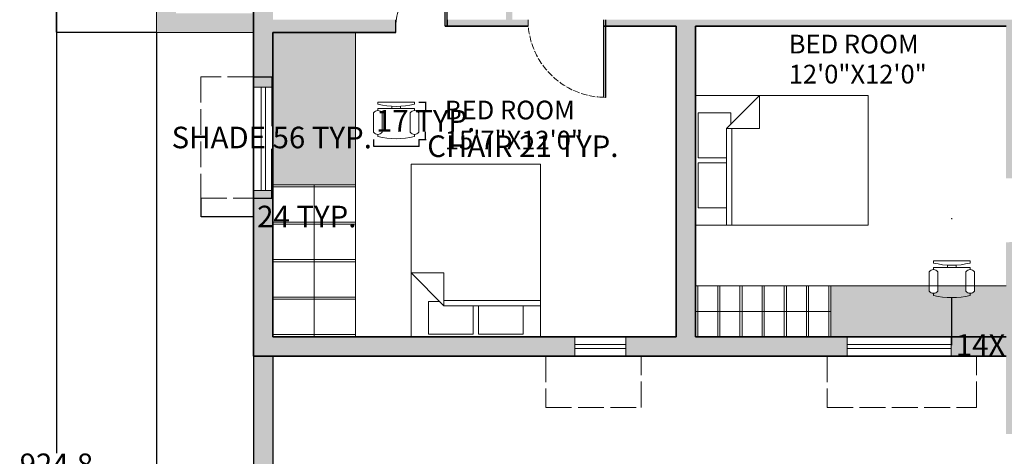
# Model space of a CAD drawing. Units: inches. Extents: x 215 to 969, y -612 to 418.
# Tile 4 of 8: x 227 to 684, y -93 to 109. Entities that reach past the tile are written whole.
import ezdxf

# ---------------------------------------------------------------- set-up
doc = ezdxf.new("R2010")
doc.units = ezdxf.units.IN
doc.header["$MEASUREMENT"] = 0
doc.linetypes.add('ACAD_ISO02W100', pattern=[15, 12, -3])
for name, color, linetype, lineweight in [('A-ANNO-DIMS', 2, 'Continuous', 18), ('A-AREA-IDEN', 7, 'Continuous', 18), ('A-DOOR', 3, 'Continuous', 25), ('A-DOOR-SWNG', 3, 'ACAD_ISO02W100', 13), ('A-FLOR-CASE', 9, 'Continuous', 18), ('A-FLOR-OVHD', 8, 'ACAD_ISO02W100', 13), ('A-FLOR-SHFT', 9, 'Continuous', 18), ('A-FLOR-SLAB', 7, 'Continuous', 25), ('A-FURN', 8, 'Continuous', 18), ('A-GLAZ', 4, 'Continuous', 18), ('A-WALL', 7, 'Continuous', 35)]:
    doc.layers.add(name, color=color, linetype=linetype, lineweight=lineweight)
doc.layers.add('A-WALL-PATT', color=252, linetype='Continuous', lineweight=13, true_color=0x939598)
doc.styles.get("Standard").update_dxf_attribs({"font": 'arial.ttf'})
doc.dimstyles.get("Standard").update_dxf_attribs({"dimtxt": 10, "dimasz": 0.18, "dimexe": 0.18, "dimexo": 0.0625, "dimgap": 0.09, "dimtad": 0, "dimtih": 1, "dimtoh": 1, "dimdec": 0, "dimzin": 0, "dimdsep": 46, "dimlunit": 3, "dimtxsty": 'Standard', "dimcen": 0.09, "dimadec": 0, "dimazin": 0, "dimtfac": 1, "dimtdec": 0, "dimtofl": 0, "dimtmove": 0, "dimatfit": 3, "dimfxl": 1, "dimtolj": 1, "dimtzin": 0, "dimarcsym": 0})

# ---------------------------------------------------------------- blocks, each defined once
blk = doc.blocks.new('Bed - Queen')
for p, q in [((0, -80.00003), (0, 0)), ((0, 0), (59.99999, 0)), ((59.99999, 0), (59.99999, -80.00003)), ((7.99999, -1.2), (28.79998, -1.2)), ((7.99999, -14.4), (7.99999, -1.2)), ((28.79998, -1.2), (28.79998, -14.4)), ((31.19999, -1.2), (51.99999, -1.2)), ((31.19999, -14.4), (31.19999, -1.2)), ((51.99999, -1.2), (51.99999, -16.4)), ((0, -14.4), (44.8, -14.4)), ((44.8, -16.8), (0, -16.8)), ((59.99999, -29.6), (44.8, -14.4)), ((44.8, -14.4), (44.8, -29.6)), ((51.99999, -16.4), (46.79936, -16.4)), ((44.8, -29.6), (59.99999, -29.6)), ((59.99999, -80.00003), (0, -80.00003))]:
    blk.add_line(p, q)
blk = doc.blocks.new('Chair - Desk')
for p, q in [((-8.5, 0), (-8.5, -1)), ((-8.5, 0), (8.5, 0)), ((8.5, 0), (8.5, -1)), ((-8.5, -3), (-8.5, -4)), ((-8.5, -3), (8.5, -3)), ((-2, -3), (-2, -1.9355)), ((2, -1.9576), (2, -3)), ((8.5, -3), (8.5, -4)), ((-10.5, -5), (-10.5, -14)), ((-6.5, -14), (-6.5, -5)), ((6.5, -5), (6.5, -14)), ((10.5, -14), (10.5, -5)), ((-8.5, -15), (-8.5, -16)), ((8.5, -15), (8.5, -16))]:
    blk.add_line(p, q)
for centre, radius, start, end in [((-8.5, -6.5), 2.5, 36.8699, 143.1301), ((0, 34.625), 36.625, 256.5803, 283.4197), ((8.5, -6.5), 2.5, 36.8699, 143.1301), ((-8.5, -12.5), 2.5, 216.8699, 323.1301), ((0, 19.625), 36.625, 256.5803, 283.4197), ((8.5, -12.5), 2.5, 216.8699, 323.1301)]:
    blk.add_arc(centre, radius, start, end)
blk = doc.blocks.new('WINDOW-SHADE-56')
for p, q in [((24.46, 56.34), (0, 56.34)), ((0, 56.34), (0, 0)), ((0, 0), (24.46, 0))]:
    blk.add_line(p, q)
blk = doc.blocks.new('WIN-FRAME-24A')
for p, q in [((0, 0), (0, 9)), ((23.77, 5.5), (0, 5.5)), ((23.77, 0), (23.77, 9)), ((0, 4.5), (0, 0)), ((23.77, 3.5), (0, 3.5))]:
    blk.add_line(p, q)
blk = doc.blocks.new('WIN-FRAME-48')
for p, q in [((0, 4.5), (0, 9)), ((0, 9), (0, 0)), ((48.04, 5.5), (0, 5.5)), ((48.04, 0), (48.04, 9)), ((48.04, 3.5), (0, 3.5))]:
    blk.add_line(p, q)
blk = doc.blocks.new('*D21')
at = {"layer": 'A-ANNO-DIMS', "color": 0, "lineweight": -2, "transparency": 16777216}
for p, q in [((391.01, 53.65), (391.01, 50.38)), ((391.19, 50.56), (411.83, 50.56)), ((412.01, 53.65), (412.01, 50.38)), ((412.01, 50.56), (412.19, 50.56))]:
    blk.add_line(p, q, dxfattribs=at)
at = {"layer": 'A-ANNO-DIMS', "color": 0, "transparency": 16777216}
for points in [[(391.19, 50.59), (391.19, 50.53), (391.01, 50.56)], [(411.83, 50.59), (411.83, 50.53), (412.01, 50.56)]]:
    blk.add_solid(points, dxfattribs=at)
at = {"layer": 'Defpoints', "color": 0, "transparency": 16777216}
for p in [(391.01, 53.71), (412.01, 53.71), (412.01, 50.56)]:
    blk.add_point(p, dxfattribs=at)
at = {"layer": 'A-ANNO-DIMS', "color": 0, "transparency": 16777216, "insert": (460.24, 50.56), "char_height": 10, "attachment_point": 5}
blk.add_mtext('\\A1;CHAIR 21 TYP.', dxfattribs=at)
blk = doc.blocks.new('*D22')
at = {"layer": 'A-ANNO-DIMS', "color": 0, "lineweight": -2, "transparency": 16777216}
for p, q in [((412.08, 71.05), (415.34, 71.05)), ((415.16, 70.87), (415.16, 67.49)), ((415.16, 53.89), (415.16, 57.27)), ((412.08, 53.71), (415.34, 53.71))]:
    blk.add_line(p, q, dxfattribs=at)
at = {"layer": 'A-ANNO-DIMS', "color": 0, "transparency": 16777216}
for points in [[(415.13, 70.87), (415.19, 70.87), (415.16, 71.05)], [(415.13, 53.89), (415.19, 53.89), (415.16, 53.71)]]:
    blk.add_solid(points, dxfattribs=at)
at = {"layer": 'Defpoints', "color": 0, "transparency": 16777216}
for p in [(412.01, 71.05), (415.16, 71.05), (412.01, 53.71)]:
    blk.add_point(p, dxfattribs=at)
at = {"layer": 'A-ANNO-DIMS', "color": 0, "transparency": 16777216, "insert": (415.16, 62.38), "char_height": 10, "attachment_point": 5}
blk.add_mtext('\\A1;17 TYP.', dxfattribs=at)
blk = doc.blocks.new('*D57')
at = {"layer": 'A-ANNO-DIMS', "color": 0, "lineweight": -2, "transparency": 16777216}
for p, q in [((335.42, 82.77), (343.98, 82.77)), ((343.8, 82.59), (343.8, 59.86)), ((343.8, 26.61), (343.8, 49.34)), ((335.42, 26.43), (343.98, 26.43))]:
    blk.add_line(p, q, dxfattribs=at)
at = {"layer": 'A-ANNO-DIMS', "color": 0, "transparency": 16777216}
for points in [[(343.77, 82.59), (343.83, 82.59), (343.8, 82.77)], [(343.77, 26.61), (343.83, 26.61), (343.8, 26.43)]]:
    blk.add_solid(points, dxfattribs=at)
at = {"layer": 'Defpoints', "color": 0, "transparency": 16777216}
for p in [(335.35, 82.77), (343.8, 82.77), (335.35, 26.43)]:
    blk.add_point(p, dxfattribs=at)
at = {"layer": 'A-ANNO-DIMS', "color": 0, "transparency": 16777216, "insert": (343.8, 54.6), "char_height": 10, "attachment_point": 5}
blk.add_mtext('\\A1;SHADE 56 TYP.', dxfattribs=at)
blk = doc.blocks.new('*D58')
at = {"layer": 'A-ANNO-DIMS', "color": 0, "lineweight": -2, "transparency": 16777216}
for p, q in [((310.89, 26.37), (310.89, 17.8)), ((335.35, 26.37), (335.35, 17.8)), ((311.07, 17.98), (335.17, 17.98)), ((335.35, 17.98), (335.53, 17.98))]:
    blk.add_line(p, q, dxfattribs=at)
at = {"layer": 'A-ANNO-DIMS', "color": 0, "transparency": 16777216}
for points in [[(311.07, 18.01), (311.07, 17.95), (310.89, 17.98)], [(335.17, 18.01), (335.17, 17.95), (335.35, 17.98)]]:
    blk.add_solid(points, dxfattribs=at)
at = {"layer": 'Defpoints', "color": 0, "transparency": 16777216}
for p in [(310.89, 26.43), (335.35, 26.43), (335.35, 17.98)]:
    blk.add_point(p, dxfattribs=at)
at = {"layer": 'A-ANNO-DIMS', "color": 0, "transparency": 16777216, "insert": (360.05, 17.98), "char_height": 10, "attachment_point": 5}
blk.add_mtext('\\A1;24 TYP.', dxfattribs=at)
blk = doc.blocks.new('*D74')
at = {"layer": 'A-ANNO-DIMS', "color": 0, "lineweight": -2, "transparency": 16777216}
for p, q in [((290.29, 181.21), (243.77, 181.21)), ((243.95, 181.03), (243.95, 147.41)), ((243.95, 103.39), (243.95, 137.02)), ((290.29, 103.21), (243.77, 103.21))]:
    blk.add_line(p, q, dxfattribs=at)
at = {"layer": 'A-ANNO-DIMS', "color": 0, "transparency": 16777216}
for points in [[(243.92, 181.03), (243.98, 181.03), (243.95, 181.21)], [(243.92, 103.39), (243.98, 103.39), (243.95, 103.21)]]:
    blk.add_solid(points, dxfattribs=at)
at = {"layer": 'Defpoints', "color": 0, "transparency": 16777216}
for p in [(243.95, 181.21), (290.35, 181.21), (290.35, 103.21)]:
    blk.add_point(p, dxfattribs=at)
at = {"layer": 'A-ANNO-DIMS', "color": 0, "transparency": 16777216, "insert": (243.95, 142.21), "char_height": 10, "attachment_point": 5}
blk.add_mtext('\\A1;78', dxfattribs=at)
blk = doc.blocks.new('*D75')
at = {"layer": 'A-ANNO-DIMS', "color": 0, "lineweight": -2, "transparency": 16777216}
for p, q in [((290.35, 103.15), (290.35, -605.89)), ((879.35, -534.51), (879.35, -605.89)), ((290.53, -605.71), (573.71, -605.71)), ((879.17, -605.71), (596, -605.71))]:
    blk.add_line(p, q, dxfattribs=at)
at = {"layer": 'A-ANNO-DIMS', "color": 0, "transparency": 16777216}
for points in [[(290.53, -605.68), (290.53, -605.74), (290.35, -605.71)], [(879.17, -605.68), (879.17, -605.74), (879.35, -605.71)]]:
    blk.add_solid(points, dxfattribs=at)
at = {"layer": 'Defpoints', "color": 0, "transparency": 16777216}
for p in [(290.35, 103.21), (879.35, -534.45), (879.35, -605.71)]:
    blk.add_point(p, dxfattribs=at)
at = {"layer": 'A-ANNO-DIMS', "color": 0, "transparency": 16777216, "insert": (584.85, -605.71), "char_height": 10, "attachment_point": 5}
blk.add_mtext('\\A1;589', dxfattribs=at)
blk = doc.blocks.new('*D76')
at = {"layer": 'A-ANNO-DIMS', "color": 0, "lineweight": -2, "transparency": 16777216}
for p, q in [((569.29, 365.5), (243.77, 365.5)), ((243.95, 365.32), (243.95, -91.71)), ((243.95, -559.13), (243.95, -102.1)), ((454.66, -559.31), (243.77, -559.31))]:
    blk.add_line(p, q, dxfattribs=at)
at = {"layer": 'A-ANNO-DIMS', "color": 0, "transparency": 16777216}
for points in [[(243.92, 365.32), (243.98, 365.32), (243.95, 365.5)], [(243.92, -559.13), (243.98, -559.13), (243.95, -559.31)]]:
    blk.add_solid(points, dxfattribs=at)
at = {"layer": 'Defpoints', "color": 0, "transparency": 16777216}
for p in [(569.35, 365.5), (243.95, -559.31), (454.72, -559.31)]:
    blk.add_point(p, dxfattribs=at)
at = {"layer": 'A-ANNO-DIMS', "color": 0, "transparency": 16777216, "insert": (243.95, -96.91), "char_height": 10, "attachment_point": 5}
blk.add_mtext('\\A1;924.8', dxfattribs=at)
blk = doc.blocks.new('*D85')
at = {"layer": 'A-ANNO-DIMS', "color": 0, "lineweight": -2, "transparency": 16777216}
for p, q in [((397.96, 133.26), (398.14, 133.26)), ((398.14, 133.26), (408.16, 123.3)), ((425.11, 106.37), (425.29, 106.37)), ((425.2, 106.28), (425.2, 106.46))]:
    blk.add_line(p, q, dxfattribs=at)
at = {"layer": 'A-ANNO-DIMS', "color": 0, "transparency": 16777216}
blk.add_solid([(408.18, 123.32), (408.14, 123.28), (408.29, 123.18)], dxfattribs=at)
at = {"layer": 'Defpoints', "color": 0, "transparency": 16777216}
for p in [(408.29, 123.18), (425.2, 106.37)]:
    blk.add_point(p, dxfattribs=at)
at = {"layer": 'A-ANNO-DIMS', "color": 0, "transparency": 16777216, "insert": (372.32, 133.26), "char_height": 10, "attachment_point": 5}
blk.add_mtext('\\A1;R23.847', dxfattribs=at)
blk = doc.blocks.new('*D94')
at = {"layer": 'A-ANNO-DIMS', "color": 0, "lineweight": -2, "transparency": 16777216}
for p, q in [((659.08, 17.02), (659.26, 17.02)), ((659.17, 16.93), (659.17, 17.11)), ((659.17, -41.58), (659.17, -19.78)), ((659.35, -41.58), (659.17, -41.58))]:
    blk.add_line(p, q, dxfattribs=at)
at = {"layer": 'A-ANNO-DIMS', "color": 0, "transparency": 16777216}
blk.add_solid([(659.2, -19.78), (659.14, -19.78), (659.17, -19.6)], dxfattribs=at)
at = {"layer": 'Defpoints', "color": 0, "transparency": 16777216}
for p in [(659.17, 17.02), (659.17, -19.6)]:
    blk.add_point(p, dxfattribs=at)
at = {"layer": 'A-ANNO-DIMS', "color": 0, "transparency": 16777216, "insert": (699.18, -41.58), "char_height": 10, "attachment_point": 5}
blk.add_mtext('\\A1;14X R36.625', dxfattribs=at)

msp = doc.modelspace()

# ---------------------------------------------------------------- hatches: boundary and pattern name
at = {"layer": 'A-WALL-PATT'}
h = msp.add_hatch(color=256, dxfattribs=at)
h.dxf.hatch_style = 1
h.paths.add_polyline_path([(764.0736, 322.2135), (569.3535, 322.2135), (565.0643, 322.2135), (565.0643, 313.2135), (569.3535, 313.2135), (569.3535, 205.2135), (509.3535, 205.2135), (509.3535, 247.2592), (506.3535, 247.2592), (506.3535, 172.2135), (491.3535, 172.2135), (491.3535, 169.2135), (509.3535, 169.2135), (509.3535, 202.2135), (569.3535, 202.2135), (569.3535, 169.2135), (578.3535, 169.2135), (578.3535, 205.2135), (578.3535, 237.2135), (615.7789, 237.2135), (615.7789, 246.2135), (578.3535, 246.2135), (578.3535, 313.2135), (710.3535, 313.2135), (710.3535, 246.2135), (710.3535, 211.3874), (719.3535, 211.3874), (719.3535, 295.2135), (719.3535, 313.2135), (764.0736, 313.2135)])
h.paths.add_polyline_path([(879.3535, 322.2135), (811.6486, 322.2135), (811.6486, 313.2135), (870.3535, 313.2135), (870.3535, 215.3905, -0.06325422), (879.3535, 216.5337), (879.3535, 313.2135)])
h.paths.add_polyline_path([(879.3535, 157.2135), (879.3535, 180.5337), (870.3535, 180.5337), (870.3535, 157.2135), (719.3535, 157.2135), (710.3535, 157.2135), (710.3535, 148.2135), (719.3535, 148.2135), (870.3535, 148.2135), (870.3535, 16.2135), (838.4933, 16.2135), (838.4933, 13.2135), (870.3535, 13.2135), (870.3535, -37.7865), (844.0345, -37.7865), (844.0345, -46.7865), (870.3535, -46.7865), (879.3535, -46.7865), (879.3535, -37.7865), (879.3535, 137.613)])
h.paths.add_polyline_path([(710.3535, 246.2135), (663.4146, 246.2135), (663.4146, 237.2135), (710.3535, 237.2135)], flags=17)
h.paths.add_polyline_path([(541.2942, 322.2135), (509.3535, 322.2135), (468.3222, 322.2135), (468.3222, 313.2135), (500.3535, 313.2135), (509.3535, 313.2135), (541.2942, 313.2135)])
h.paths.add_polyline_path([(509.3535, 313.2135), (503.3535, 313.2135), (503.3535, 277.5241, -0.04952579), (509.3535, 277.4203)], flags=17)
h.paths.add_polyline_path([(420.2828, 322.2135), (335.3535, 322.2135), (335.3535, 235.2487), (344.3535, 235.2487), (344.3535, 284.1885), (344.3535, 313.2135), (420.2828, 313.2135)])
h.paths.add_polyline_path([(335.3535, 181.2135), (290.3535, 181.2135), (290.3535, 103.2135), (335.3535, 103.2135), (335.3535, 112.2135), (299.3535, 112.2135), (299.3535, 129.1615), (299.3535, 172.2135), (335.3535, 172.2135)])
h.paths.add_polyline_path([(344.3535, 199.3097), (335.3535, 199.3097), (335.3535, 172.2135), (335.3535, 157.3369), (344.3535, 157.3369), (344.3535, 169.2135), (452.3535, 169.2135), (452.5037, 169.2135), (452.5037, 150.1199), (452.3535, 109.2135), (455.3535, 109.2135), (455.3535, 169.2135, -0.02086055), (455.4787, 172.2135), (344.3535, 172.2135)])
h.paths.add_polyline_path([(344.3535, 133.3441), (335.3535, 133.3441), (335.3535, 77.89), (344.3535, 77.89), (344.3535, 103.2135), (401.3556, 103.2135), (401.3556, 109.2135), (344.3535, 109.2135)])
h.paths.add_polyline_path([(462.6362, 109.2135), (443.0437, 109.2135), (425.2018, 109.2135), (425.2018, 106.2135), (452.3535, 106.2135), (462.7615, 106.2135, -0.02086055)])
h.paths.add_polyline_path([(540.3535, 106.2135), (684.3535, 106.2135), (684.3535, 35.7135), (687.3535, 35.7135), (687.3535, 56.1856), (693.3535, 56.1856), (693.3535, 109.2135), (540.3535, 109.2135), (531.3535, 109.2135), (498.6362, 109.2135), (498.6362, 106.2135), (531.3535, 106.2135), (531.3535, -37.7865), (507.9524, -37.7865), (507.9524, -46.7865), (610.6038, -46.7865), (610.6038, -37.7865), (540.3535, -37.7865)])
h.paths.add_polyline_path([(578.3535, 358.6622), (555.879, 358.6622), (555.879, 349.6622), (569.3535, 349.6622), (569.3535, 322.2135), (578.3535, 322.2135)])
h.paths.add_polyline_path([(525.962, 358.6622), (503.3535, 358.6622), (503.3535, 322.2135), (509.3535, 322.2135), (509.3535, 349.6622), (525.962, 349.6622)])
h.paths.add_polyline_path([(344.3535, 30.022), (335.3535, 30.022), (335.3535, -37.7865), (335.3535, -46.7865), (484.3302, -46.7865), (484.3302, -37.7865), (344.3535, -37.7865)])
h.paths.add_polyline_path([(719.1188, -37.7865), (698.4193, -37.7865), (693.3535, -37.7865), (693.3535, 7.424, -0.07717369), (684.3535, 6.0404), (684.3535, -37.7865), (658.8269, -37.7865), (658.8269, -46.7865), (684.3535, -46.7865), (684.3535, -82.7865), (693.3535, -82.7865), (704.1236, -82.7865), (704.1236, -78.0462), (693.3535, -78.0462), (693.3535, -46.7865), (719.1188, -46.7865)])
h.paths.add_polyline_path([(684.3535, -14.2202), (669.6716, -14.2202), (669.6716, -16.6044, -0.23606798), (667.6716, -17.6044), (667.6716, -18.6044, -0.11764706), (650.6716, -18.6044), (650.6716, -17.6044, -0.23606798), (648.6716, -16.6044), (648.6716, -14.2202), (603.0565, -14.2202), (603.0565, -37.7865), (684.3535, -37.7865)], flags=17)
h.paths.add_polyline_path([(665.6716, -14.2202), (652.6716, -14.2202), (652.6716, -16.6044, -0.23606798), (650.6716, -17.6044), (650.6716, -18.6044, 0.11764706), (667.6716, -18.6044), (667.6716, -17.6044, -0.23606798), (665.6716, -16.6044)], flags=16)
h.paths.add_polyline_path([(786.7385, -37.7865), (755.3535, -37.7865), (755.3535, 13.2135), (769.0808, 13.2135), (769.0808, 16.2135), (755.3535, 16.2135), (755.3535, 73.2135), (753.3535, 73.2135), (693.3535, 73.2135), (693.3535, 70.2135), (753.3535, 70.2135), (753.3535, -37.7865), (743.3062, -37.7865), (743.3062, -46.7865), (781.7385, -46.7865), (781.7385, -82.7865), (786.7385, -82.7865), (786.7385, -82.3744), (786.7385, -46.7865)])
h.paths.add_polyline_path([(844.0345, -37.7865), (786.7385, -37.7865), (786.7385, -46.7865), (844.0345, -46.7865)], flags=17)
h.paths.add_polyline_path([(781.7385, -78.0462), (704.1236, -78.0462), (704.1236, -82.7865), (781.7385, -82.7865)], flags=17)
h.paths.add_polyline_path([(344.3535, -46.7865), (335.3535, -46.7865), (335.3535, -166.4525), (344.3535, -166.4525)])
h.paths.add_polyline_path([(382.6632, 103.2135), (344.3535, 103.2135), (344.3535, 77.89), (344.3535, 32.7135), (363.5083, 32.7135), (382.6632, 32.7135)])
h.paths.add_polyline_path([(879.3535, -46.7865), (870.3535, -46.7865), (870.3535, -166.4525), (879.3535, -166.4525)])
h.paths.add_polyline_path([(879.3535, -166.4525), (799.4745, -166.4525), (799.4745, -175.4525), (855.3535, -175.4525), (870.3535, -175.4525), (870.3535, -192.5449), (879.3535, -192.5449), (879.3535, -175.4525)])
h.paths.add_polyline_path([(763.1775, -166.4525), (655.7214, -166.4525), (655.7214, -175.4525), (763.1775, -175.4525)])
h.paths.add_polyline_path([(619.8538, -166.4525), (550.8369, -166.4525), (550.8369, -175.4525), (619.8538, -175.4525)])
h.paths.add_polyline_path([(527.1282, -166.4525), (427.0819, -166.4525), (427.0819, -175.4525), (527.1282, -175.4525)])
h.paths.add_polyline_path([(391.4021, -166.4525), (335.3535, -166.4525), (335.3535, -175.4525), (335.3535, -236.0109), (344.3535, -236.0109), (344.3535, -187.5037), (344.3535, -175.4525), (391.4021, -175.4525)])
h.paths.add_polyline_path([(344.3535, -271.9249), (335.3535, -271.9249), (335.3535, -331.0209), (344.3535, -331.0209), (344.3535, -314.4525), (412.4218, -314.4525, -0.02503209), (412.3073, -311.4525), (344.3535, -311.4525)])
h.paths.add_polyline_path([(470.1954, -311.4525), (442.3073, -311.4525), (442.3073, -314.4525), (470.0702, -314.4525, -0.02086055)])
h.paths.add_polyline_path([(455.3535, -314.4525), (452.3535, -314.4525), (452.3535, -374.4525), (455.3535, -374.4525)])
h.paths.add_polyline_path([(579.3535, -241.4072), (519.3535, -241.4072), (519.3535, -283.4525), (579.3535, -283.4525)])
h.paths.add_polyline_path([(516.5043, -281.1089), (584.3098, -281.1089), (584.3098, -264.0138), (516.5043, -264.0138)], flags=9)
h.paths.add_polyline_path([(516.4662, -263.2183), (581.1504, -263.2183), (581.1504, -245.8948), (516.4662, -245.8948)], flags=9)

# ---------------------------------------------------------------- linework, layer by layer
at = {"layer": 'A-DOOR'}
for p, q in [((424.2018, 106.2135), (424.2018, 130.2135)), ((425.2018, 106.2135), (425.2018, 130.2135)), ((401.3556, 103.2135), (401.3556, 109.2135)), ((425.2018, 106.2135), (424.2018, 106.2135)), ((425.2018, 109.2135), (425.2018, 106.2135)), ((497.6362, 109.2135), (497.6362, 73.2135)), ((498.6362, 109.2135), (498.6362, 73.2135))]:
    msp.add_line(p, q, dxfattribs=at)
at = {"layer": 'A-DOOR-SWNG'}
msp.add_arc((425.2018, 106.3669), 23.8466, 90, 180.368506, dxfattribs=at)
at = {"layer": 'A-DOOR-SWNG', "ltscale": 0.25}
msp.add_arc((498.6362, 109.2135), 36, 180, 270, dxfattribs=at)
at = {"layer": 'A-FLOR-CASE'}
for p, q in [((382.6632, 103.2135), (382.6632, -37.7865)), ((382.6632, 32.7135), (344.3535, 32.7135)), ((344.3535, 32.7135), (363.5083, 32.7135)), ((363.5083, 32.7135), (363.5083, -37.7865)), ((382.6632, 32.7135), (382.6632, 31.7135)), ((382.6632, 31.7135), (344.3535, 31.7135)), ((382.6632, 15.3497), (344.3535, 15.3497)), ((344.3535, 15.3497), (363.5083, 15.3497)), ((382.6632, 14.3497), (344.3535, 14.3497)), ((382.6632, -2.0142), (344.3535, -2.0142)), ((344.3535, -2.0142), (363.5083, -2.0142)), ((382.6632, -3.0142), (344.3535, -3.0142)), ((344.3535, -14.2202), (344.3535, -37.7865)), ((531.3535, -37.7865), (531.3535, -14.2202)), ((684.3535, -14.2202), (540.3535, -14.2202)), ((541.3535, -37.7865), (541.3535, -14.2202)), ((550.6373, -14.2202), (550.6373, -37.7865)), ((551.6373, -37.7865), (551.6373, -14.2202)), ((560.9212, -14.2202), (560.9212, -37.7865)), ((561.9212, -37.7865), (561.9212, -14.2202)), ((571.205, -14.2202), (571.205, -37.7865)), ((572.205, -37.7865), (572.205, -14.2202)), ((581.4889, -14.2202), (581.4889, -37.7865)), ((582.4889, -37.7865), (582.4889, -14.2202)), ((591.7727, -14.2202), (591.7727, -37.7865)), ((592.7727, -37.7865), (592.7727, -14.2202)), ((602.0565, -14.2202), (602.0565, -37.7865)), ((603.0565, -37.7865), (603.0565, -14.2202)), ((382.6632, -19.3781), (344.3535, -19.3781)), ((344.3535, -19.3781), (363.5083, -19.3781)), ((382.6632, -20.3781), (344.3535, -20.3781)), ((603.0565, -26.0033), (540.3535, -26.0033)), ((382.6632, -36.742), (344.3535, -36.742)), ((344.3535, -36.742), (363.5083, -36.742)), ((382.6632, -37.742), (344.3535, -37.742)), ((344.3535, -37.7865), (345.3535, -37.7865))]:
    msp.add_line(p, q, dxfattribs=at)
at = {"layer": 'A-FLOR-OVHD'}
for p, q in [((470.8332, -46.7865), (470.8332, -70.5745)), ((515.1767, -70.5745), (515.1767, -46.7865)), ((601.3609, -46.7865), (601.3609, -70.5864)), ((670.6794, -70.5864), (670.6794, -46.7865)), ((470.8332, -70.5745), (515.1767, -70.5745)), ((601.3609, -70.5864), (670.6794, -70.5864))]:
    msp.add_line(p, q, dxfattribs=at)
at = {"layer": 'A-FLOR-SHFT'}
for p, q in [((290.3535, 181.2135), (290.3535, 103.2135)), ((290.3535, 103.2135), (335.3535, 103.2135))]:
    msp.add_line(p, q, dxfattribs=at)
at = {"layer": 'A-FLOR-SLAB'}
for p, q in [((335.3535, -46.7865), (335.3535, -175.4525)), ((344.3535, -46.7865), (344.3535, -166.4525))]:
    msp.add_line(p, q, dxfattribs=at)
at = {"layer": 'A-WALL'}
for p, q in [((335.3535, -37.7865), (335.3535, 172.2135)), ((335.3535, 106.2135), (335.3535, -37.7865)), ((424.2018, 106.2135), (452.3535, 106.2135)), ((462.7615, 106.2135), (443.0437, 106.2135)), ((531.3535, 106.2135), (497.6362, 106.2135)), ((531.3535, -37.7865), (531.3535, 106.2135)), ((540.3535, -37.7865), (540.3535, 106.2135)), ((540.3535, 106.2135), (684.3535, 106.2135)), ((344.3535, 103.2135), (401.3556, 103.2135)), ((344.3535, 103.2135), (344.3535, -37.7865)), ((335.3535, -46.7865), (335.3535, -37.7865)), ((344.3535, -37.7865), (531.3535, -37.7865)), ((684.3535, -37.7865), (540.3535, -37.7865)), ((684.3535, -46.7865), (335.3535, -46.7865)), ((344.3535, -46.7865), (531.3535, -46.7865)), ((684.3535, -46.7865), (540.3535, -46.7865))]:
    msp.add_line(p, q, dxfattribs=at)

# ---------------------------------------------------------------- block references
at = {"layer": 'A-FLOR-OVHD'}
msp.add_blockref('WINDOW-SHADE-56', (310.895, 26.4314), dxfattribs=at)
at = {"layer": 'A-FURN'}
for p, rotation in [((540.3535, 14.0216), 89.99999999999962), ((468.4217, -37.7865), 180)]:
    msp.add_blockref('Bed - Queen', p, dxfattribs=dict(at, rotation=rotation))
for p in [(401.5147, 71.0474), (659.1716, -2.6044)]:
    msp.add_blockref('Chair - Desk', p, dxfattribs=at)
at = {"layer": 'A-GLAZ', "extrusion": (0, 0, -1), "zscale": -1}
for name, p, xscale, rotation in [('WIN-FRAME-48', (-335.3539, 30.0222), 0.996431308931832, 90), ('WIN-FRAME-24A', (-484.33, -37.7869), 0.9937777459029128, 179.9999991462263), ('WIN-FRAME-48', (-610.604, -37.7869), 1.003824078718851, 180)]:
    msp.add_blockref(name, p, dxfattribs=dict(at, xscale=xscale, rotation=rotation))

# ---------------------------------------------------------------- texts
at = {"layer": 'A-AREA-IDEN'}
for s, height, p in [('BED ROOM', 8.67737, (583.5517, 93.5721)), ('12\'0"X12\'0"', 8.677368, (583.5517, 79.6327)), ('BED ROOM', 8.67737, (424.0988, 62.9961)), ('15\'7"X12\'0"', 8.677368, (424.0988, 49.0567))]:
    msp.add_text(s, height=height, dxfattribs=at).set_placement(p)

# ---------------------------------------------------------------- dimensions: what is measured, and where the dimension line sits
at = {"layer": 'A-ANNO-DIMS'}
for base, p1, p2, override, picture, middle in [((243.9535, -559.3132), (569.3535, 365.5008), (454.7218, -559.3132), {"dimdec": 1, "dimlfac": 1, "dimrnd": 0, "dimzin": 0, "dimdsep": 46, "dimlunit": 2}, '*D76', (243.9535, -96.9062)), ((243.9535, 181.2135), (290.3535, 103.2135), (290.3535, 181.2135), {"dimdec": 0, "dimlfac": 1, "dimrnd": 0, "dimzin": 0, "dimdsep": 46, "dimlunit": 2}, '*D74', (243.9535, 142.2135))]:
    dim = msp.add_linear_dim(base=base, p1=p1, p2=p2, angle=90, dimstyle='Standard', override=override, dxfattribs=at)
    dim.commit()
    dim.dimension.update_dxf_attribs({"geometry": picture, "text_midpoint": middle})
dim = msp.add_radius_dim(center=(425.2018, 106.3669), mpoint=(408.2859, 123.1751), dimstyle='Standard', override={"dimdec": 3, "dimlfac": 1, "dimrnd": 0, "dimzin": 0, "dimdsep": 46, "dimlunit": 2}, dxfattribs=at)
dim.commit()
dim.dimension.update_dxf_attribs({"geometry": '*D85', "text_midpoint": (372.3241, 133.26), "dimtype": 164})
dim = msp.add_linear_dim(base=(879.3535, -605.7132), p1=(290.3535, 103.2135), p2=(879.3535, -534.4525), dimstyle='Standard', override={"dimdec": 0, "dimlfac": 1, "dimrnd": 0, "dimzin": 0, "dimdsep": 46, "dimlunit": 2}, dxfattribs=at)
dim.commit()
dim.dimension.update_dxf_attribs({"geometry": '*D75', "text_midpoint": (584.8535, -605.7132)})
for base, p1, p2, text, picture, middle in [((343.8038, 82.7669), (335.3535, 26.4318), (335.3535, 82.7669), 'SHADE <> TYP.', '*D57', (343.8038, 54.5994)), ((415.1647, 71.0474), (412.0147, 53.7141), (412.0147, 71.0474), '<> TYP.', '*D22', (415.1647, 62.3808))]:
    dim = msp.add_linear_dim(base=base, p1=p1, p2=p2, angle=90, text=text, dimstyle='Standard', override={"dimdec": 0, "dimlfac": 1, "dimrnd": 0, "dimzin": 0, "dimdsep": 46, "dimlunit": 2}, dxfattribs=at)
    dim.commit()
    dim.dimension.update_dxf_attribs({"geometry": picture, "text_midpoint": middle})
for base, p1, p2, text, picture, middle in [((412.0147, 50.5641), (391.0147, 53.7141), (412.0147, 53.7141), 'CHAIR <> TYP.', '*D21', (460.2383, 50.5641)), ((335.3535, 17.9815), (310.8946, 26.4318), (335.3535, 26.4318), '<> TYP.', '*D58', (360.0471, 17.9815))]:
    dim = msp.add_linear_dim(base=base, p1=p1, p2=p2, text=text, dimstyle='Standard', override={"dimdec": 0, "dimlfac": 1, "dimrnd": 0, "dimzin": 0, "dimdsep": 46, "dimlunit": 2}, dxfattribs=at)
    dim.commit()
    dim.dimension.update_dxf_attribs({"geometry": picture, "text_midpoint": middle})
dim = msp.add_radius_dim(center=(659.1716, 17.0206), mpoint=(659.172, -19.6044), text='14X <>', dimstyle='Standard', override={"dimdec": 3, "dimlfac": 1, "dimrnd": 0, "dimzin": 0, "dimdsep": 46, "dimlunit": 2}, dxfattribs=at)
dim.commit()
dim.dimension.update_dxf_attribs({"geometry": '*D94', "text_midpoint": (699.1796, -41.5794), "dimtype": 164})

doc.saveas('drawing.dxf')
